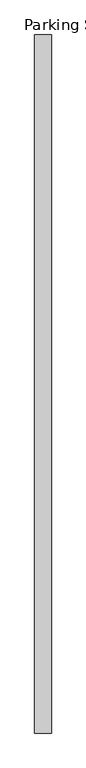
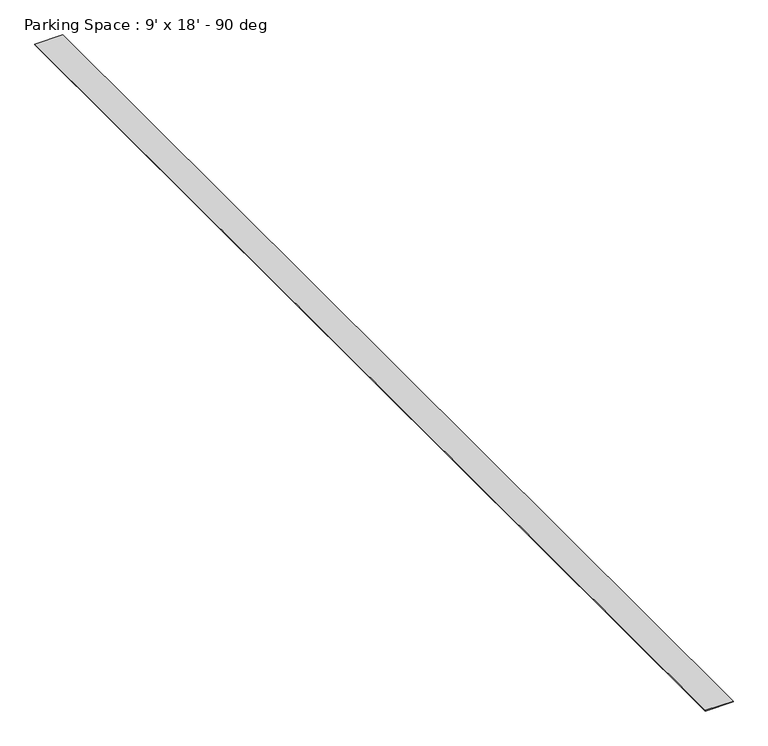
"""IFC4 building model written with IfcOpenShell, lengths in millimetres: proxy geometry, Parking Space : 9' x 18' - 90 deg."""

from ifc_helpers import new_model, si_unit, origin, origin_with_axes, place, context, project, spatial, polyline, outline, extrude, source, transform, mapped, element, save


def parking_space_9_x_18_90_deg_fdd9e8f5(model_context):
    return source(origin(), model_context, "Body", "SweptSolid", [
        extrude(outline(polyline([(-50.8, 0.0), (50.8, 0.0), (50.8, -4267.2), (-50.8, -4267.2), (-50.8, 0.0)])), origin_with_axes(), (0.0, 0.0, 1.0), 3.175),
    ])


if __name__ == "__main__":
    model = new_model("IFC4")
    model_context = context("Model", 3, world=origin())
    ifc_project = project(units=[si_unit("LENGTHUNIT", "METRE", prefix="MILLI")], contexts=[model_context])
    site = spatial("IfcSite", under=ifc_project)
    building = spatial("IfcBuilding", under=site)
    placement = place(None, origin())
    parking_space_9_x_18_90_deg_shape = parking_space_9_x_18_90_deg_fdd9e8f5(model_context)
    element("IfcBuildingElementProxy", 1, Name="Parking Space : 9' x 18' - 90 deg", ObjectType="Parking Space : 9' x 18' - 90 deg", at=placement, inside=building, context=model_context, shape_type="MappedRepresentation", body=[
        mapped(parking_space_9_x_18_90_deg_shape, transform((0.0, 0.0, 0.0), x_axis=(1.0, 0.0, 0.0), y_axis=(0.0, 1.0, 0.0), z_axis=(0.0, 0.0, 1.0))),
    ])
    save(model, "model.ifc")

# Revit data of these elements
# Type "Parking Space : 9' x 18' - 90 deg"
#   Angle = 90.00°
#   Parking Length = 18' - 0"
#   Parking Width = 9' - 0"
#   pl = 14' - 0"
#   pw = 8' - 0"
# Element 1 (IfcBuildingElementProxy, "Parking Space : 9' x 18' - 90 deg")
#   Materials on its faces: "Parking Stripe"
# Materials
#   "Parking Stripe": class "Paint", colour RGB 250 250 91, transparency 0
